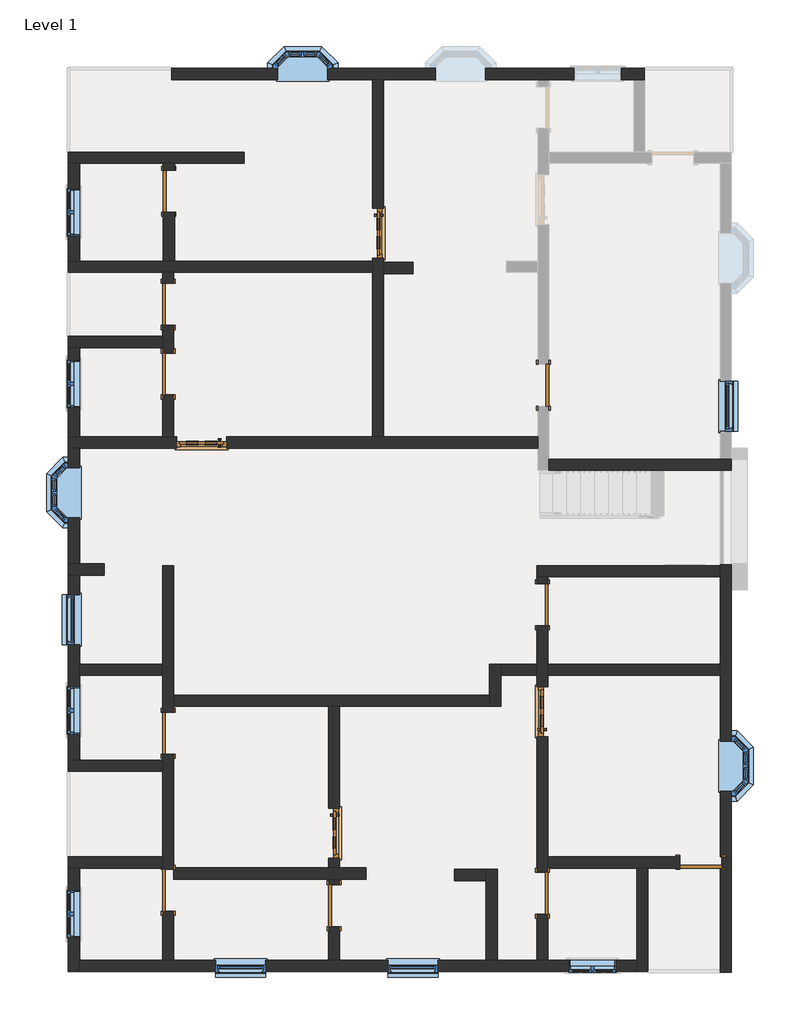
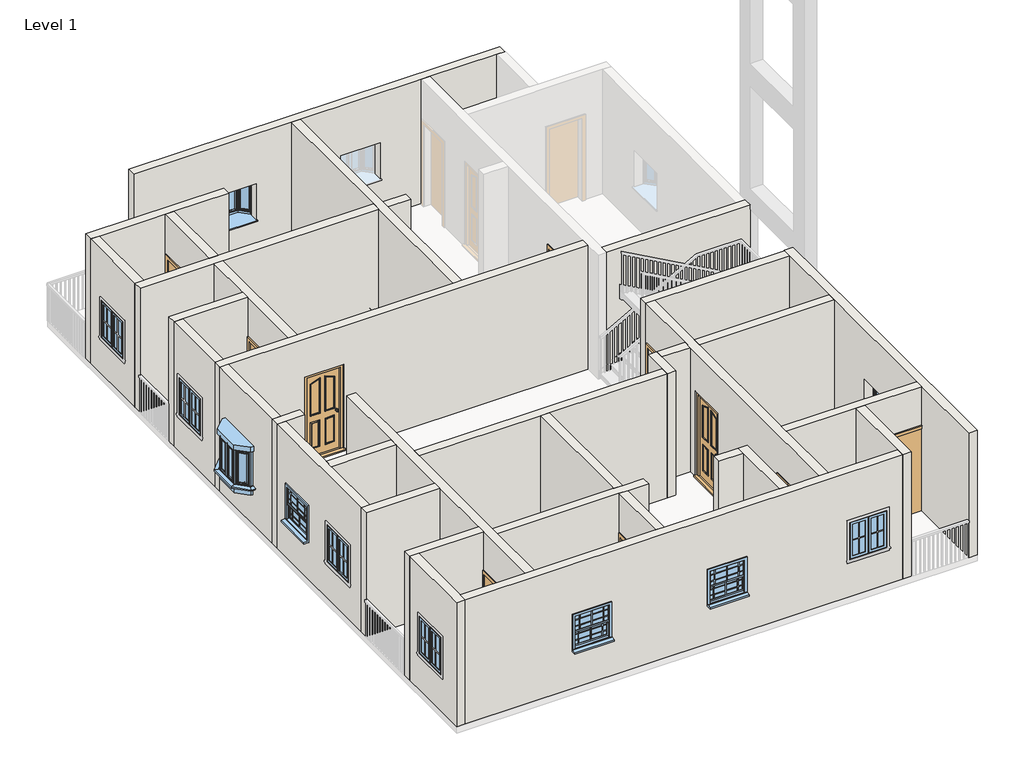
# One storey, part 1 of 4: 34 walls, 14 doors, 12 windows.
# Revit data of these elements (continued)
# Element 23 (IfcWall, "Generic - 4.5\"")
#   Top Offset = 0' - 0"
#   Base Offset = 0' - 0"
#   wall height = 10' - 0"
#   Phase Created = New Construction
#   Base Constraint = Level 1
#   Top Constraint = Level 2
#   Materials on its faces: "Default Wall", "Door - Frame/Mullion"
# Elements 24, 25, 26, 29, 32, 33, 34, 35, 36, 37, 38, 39, 40 (IfcWall, "Generic - 4.5\"")
#   Top Offset = 0' - 0"
#   Base Offset = 0' - 0"
#   wall height = 10' - 0"
#   Phase Created = New Construction
#   Base Constraint = Level 1
#   Top Constraint = Level 2
#   Materials on its faces: "Default Wall"
# Element 28 (IfcWall, "Generic - 4.5\"")
#   Top Offset = 0' - 0"
#   Base Offset = 0' - 0"
#   wall height = 10' - 0"
#   Phase Created = New Construction
#   Base Constraint = Level 1
#   Top Constraint = Level 2
#   Materials on its faces: "Default Wall", "Parking Stripe", "Cherry"
# Element 41 (IfcWall, "Generic - 9\"")
#   Top Offset = 0' - 0"
#   Base Offset = 0' - 0"
#   wall height = 10' - 0"
#   Phase Created = New Construction
#   Base Constraint = Level 1
#   Top Constraint = Level 2
#   Materials on its faces: "Default Wall", "Parking Stripe", "Earth", "Cherry"
# Element 42 (IfcWall, "Generic - 9\"")
#   Top Offset = 0' - 0"
#   Base Offset = 0' - 0"
#   wall height = 10' - 0"
#   Phase Created = New Construction
#   Base Constraint = Level 1
#   Top Constraint = Level 2
#   Materials on its faces: "Default Wall", "Door - Frame/Mullion", "Parking Stripe"
# Element 43 (IfcWall, "Generic - 9\"")
#   Top Offset = 0' - 0"
#   Base Offset = 0' - 0"
#   wall height = 10' - 0"
#   Phase Created = New Construction
#   Base Constraint = Level 1
#   Top Constraint = Level 2
#   Materials on its faces: "Default Wall", "Parking Stripe"
# Elements 44, 45, 48 (IfcWall, "Generic - 9\"")
#   Top Offset = 0' - 0"
#   Base Offset = 0' - 0"
#   wall height = 10' - 0"
#   Phase Created = New Construction
#   Base Constraint = Level 1
#   Top Constraint = Level 2
#   Materials on its faces: "Default Wall", "Earth"
# Element 46 (IfcWall, "Generic - 9\"")
#   Top Offset = 0' - 0"
#   Base Offset = 0' - 0"
#   wall height = 10' - 0"
#   Phase Created = New Construction
#   Base Constraint = Level 1
#   Top Constraint = Level 2
#   Materials on its faces: "Default Wall", "Parking Stripe", "Cherry"
# Element 47 (IfcWall, "Generic - 9\"")
#   Top Offset = 0' - 0"
#   Base Offset = 0' - 0"
#   wall height = 10' - 0"
#   Phase Created = New Construction
#   Base Constraint = Level 1
#   Top Constraint = Level 2
#   Materials on its faces: "Default Wall", "Cherry"
# Element 49 (IfcWindow, "910x910mm")
#   Mark = "1"
#   Phase Created = New Construction
#   Materials on its faces: "Window Frame", "Glass"
# Element 50 (IfcWindow, "910x910mm")
#   Mark = "4"
#   Phase Created = New Construction
#   Materials on its faces: "Window Frame", "Glass"
# Element 51 (IfcWindow, "910x910mm")
#   Mark = "5"
#   Phase Created = New Construction
#   Materials on its faces: "Window Frame", "Glass"
# Element 52 (IfcWindow, "Window-Casement-Double : 34\" x 36\"")
#   Mark = "10"
#   Window Inset = 0' - 0"
#   Interior Wall Closure = 0' - 2 1/4"
#   Frame Extension = 0' - 0 1/4"
#   Exterior Wall Closure = 0' - 1 1/4"
#   Interior Trim Visibility = yes
#   Exterior Trim Visibility = yes
#   Phase Created = New Construction
#   Materials on its faces: "Wood - Stained", "Glass", "Clad - White"
# Element 53 (IfcWindow, "Window-Casement-Double : 34\" x 36\"")
#   Mark = "11"
#   Window Inset = 0' - 0"
#   Interior Wall Closure = 0' - 2 1/4"
#   Frame Extension = 0' - 0 1/4"
#   Exterior Wall Closure = 0' - 1 1/4"
#   Interior Trim Visibility = yes
#   Exterior Trim Visibility = yes
#   Phase Created = New Construction
#   Materials on its faces: "Wood - Stained", "Glass", "Clad - White"
# Element 54 (IfcWindow, "Window-Casement-Double : 34\" x 36\"")
#   Mark = "13"
#   Window Inset = 0' - 0"
#   Interior Wall Closure = 0' - 2 1/4"
#   Frame Extension = 0' - 0 1/4"
#   Exterior Wall Closure = 0' - 1 1/4"
#   Interior Trim Visibility = yes
#   Exterior Trim Visibility = yes
#   Phase Created = New Construction
#   Materials on its faces: "Wood - Stained", "Glass", "Clad - White"
# Element 55 (IfcWindow, "Window-Casement-Double : 34\" x 36\"")
#   Mark = "14"
#   Window Inset = 0' - 0"
#   Interior Wall Closure = 0' - 2 1/4"
#   Frame Extension = 0' - 0 1/4"
#   Exterior Wall Closure = 0' - 1 1/4"
#   Interior Trim Visibility = yes
#   Exterior Trim Visibility = yes
#   Phase Created = New Construction
#   Materials on its faces: "Wood - Stained", "Glass", "Clad - White"
# Element 56 (IfcWindow, "Window-Casement-Double : 34\" x 36\"")
#   Mark = "15"
#   Window Inset = 0' - 0"
#   Interior Wall Closure = 0' - 2 1/4"
#   Frame Extension = 0' - 0 1/4"
#   Exterior Wall Closure = 0' - 1 1/4"
#   Interior Trim Visibility = yes
#   Exterior Trim Visibility = yes
#   Phase Created = New Construction
#   Materials on its faces: "Wood - Stained", "Glass", "Clad - White"
# Element 57 (IfcWindow, "Windows_Sash_w-Bars_1 : 910x910mm")
#   Mark = "6"
#   Phase Created = New Construction
#   Materials on its faces: "Window Frame", "Glass"
# Element 58 (IfcWindow, "Windows_Sash_w-Bars_1 : 910x910mm")
#   Mark = "7"
#   Phase Created = New Construction
#   Materials on its faces: "Window Frame", "Glass"
# Element 59 (IfcWindow, "Windows_Sash_w-Bars_1 : 910x910mm")
#   Mark = "8"
#   Phase Created = New Construction
#   Materials on its faces: "Window Frame", "Glass"
# Element 60 (IfcWindow, "Windows_Sash_w-Bars_1 : 910x910mm")
#   Mark = "9"
#   Phase Created = New Construction
#   Materials on its faces: "Window Frame", "Glass"
# Materials
#   "Door - Glazing": colour RGB 0 0 255, transparency 0.75
#   "Door - Panel": class "Wood", colour RGB 210 159 95, transparency 0, Cost = 0
#   "Door - Frame/Mullion": class "Wood", colour RGB 212 179 113, transparency 0
#   "Door - Handle": colour RGB 247 247 247, transparency 0
#   "Door - Frame": colour RGB 118 70 51, transparency 0, Cost = 0
#   "Window Frame": colour RGB 249 249 249, transparency 0
#   "Glass": class "Glass", colour RGB 0 128 192, transparency 0.75, Description = "Soda Lime Glass", Cost = 0
#   "Wood - Stained": class "Wood", colour RGB 224 178 126, transparency 0, Cost = 0
#   "Clad - White": class "Wood", colour RGB 242 242 238, transparency 0, Cost = 0
#   "Default Wall": colour RGB 128 128 128, transparency 0, Cost = 0
#   "Brick, Soldier Course": class "Masonry", colour RGB 170 98 104, transparency 0, Description = "Common brick soldier coursed", Cost = 0
#   "Parking Stripe": class "Paint", colour RGB 250 250 91, transparency 0, Cost = 0
#   "Earth": class "Generic", colour RGB 97 75 62, transparency 0, Description = "Soil", Cost = 0
#   "Cherry": class "Wood", colour RGB 226 177 128, transparency 0, Description = "Prunus Serotina", Cost = 0
